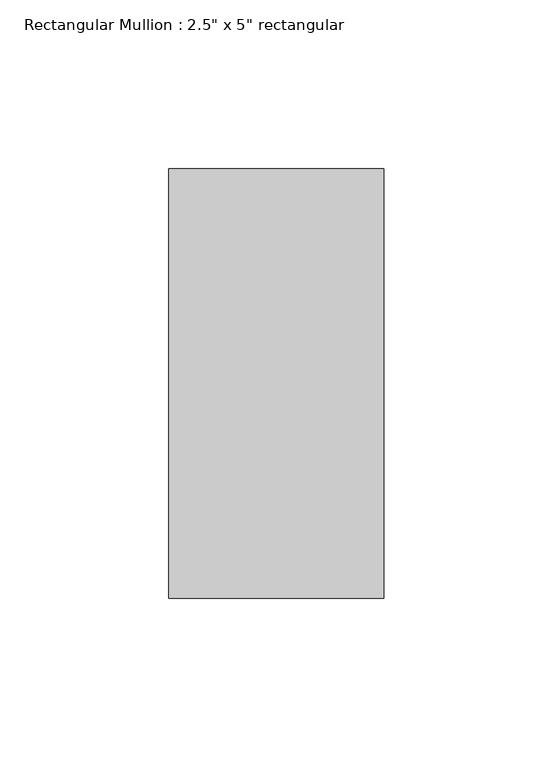
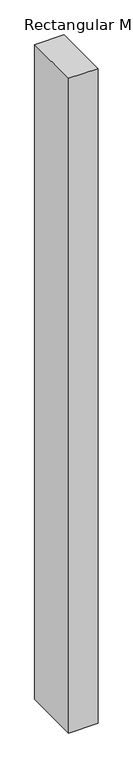
"""IFC4 building model written with IfcOpenShell, lengths in millimetres: member geometry."""

from ifc_helpers import new_model, si_unit, frame, origin, place, context, project, spatial, polyline, outline, extrude, source, transform, mapped, element, save


def member_92f7bfeb(model_context):
    return source(origin(), model_context, "Body", "SweptSolid", [
        extrude(outline(polyline([(0.0, 63.5), (0.0, -63.5), (-63.5, -63.5), (-63.5, 63.5), (0.0, 63.5)])), frame((0.0, 0.0, -1492.2228074), z_axis=(0.0, 0.0, 1.0), x_axis=(1.0, 0.0, 0.0)), (0.0, 0.0, 1.0), 1492.2228074),
    ])


if __name__ == "__main__":
    model = new_model("IFC4")
    model_context = context("Model", 3, world=origin())
    ifc_project = project(units=[si_unit("LENGTHUNIT", "METRE", prefix="MILLI")], contexts=[model_context])
    site = spatial("IfcSite", under=ifc_project)
    building = spatial("IfcBuilding", under=site)
    placement = place(None, origin())
    member_shape = member_92f7bfeb(model_context)
    element("IfcMember", 1, ObjectType="Rectangular Mullion : 2.5\" x 5\" rectangular", at=placement, inside=building, context=model_context, shape_type="MappedRepresentation", body=[
        mapped(member_shape, transform((0.0, 0.0, 0.0), x_axis=(1.0, 0.0, 0.0), y_axis=(0.0, 1.0, 0.0), z_axis=(0.0, 0.0, 1.0))),
    ])
    save(model, "model.ifc")

# Revit data of these elements
# Type "Rectangular Mullion : 2.5\" x 5\" rectangular"
#   built-in parameter 1007304 = 0.416667 (stored number, unit not read)
#   built-in parameter 1007301 = 0.104167 (stored number, unit not read)
#   built-in parameter 1007300 = 0.104167 (stored number, unit not read)
# Element 1 (IfcMember, "Rectangular Mullion : 2.5\" x 5\" rectangular")
#   Materials on its faces: "Aluminum"
# Materials
#   "Aluminum": class "Metal", colour RGB 247 247 247, transparency 0, Description = "Aluminum 6061", Cost = 0
